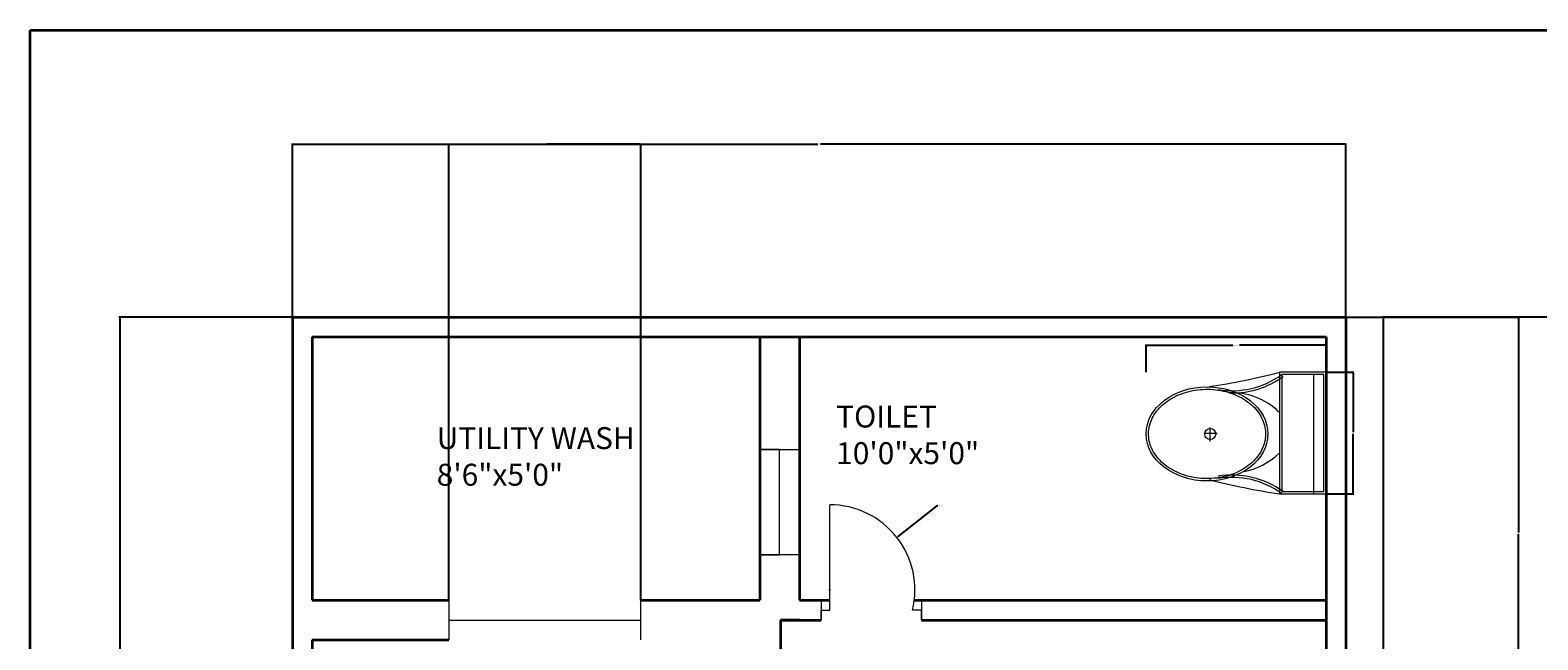
# Model space of a CAD drawing. Units: inches. Extents: x 1734 to 2405, y 1500 to 2491.
# Tile 13 of 14: x 1734 to 2078, y 2352 to 2491. Entities that reach past the tile are written whole.
import ezdxf

# ---------------------------------------------------------------- set-up
doc = ezdxf.new("R2010")
doc.units = ezdxf.units.IN
for name, color, linetype, lineweight in [('A-ANNO-DIMS', 2, 'Continuous', 18), ('A-ANNO-TTLB', 7, 'Continuous', 35), ('A-AREA-IDEN', 7, 'Continuous', 18), ('A-DOOR', 3, 'Continuous', 18), ('A-FLOR-FIXT', 9, 'Continuous', 18), ('A-GLAZ', 4, 'Continuous', 18), ('A-WALL', 7, 'Continuous', 35)]:
    doc.layers.add(name, color=color, linetype=linetype, lineweight=lineweight)
doc.styles.get("Standard").update_dxf_attribs({"font": 'arial.ttf'})
doc.dimstyles.get("Standard").update_dxf_attribs({"dimtxt": 0.18, "dimasz": 0.18, "dimexe": 0.18, "dimexo": 0.0625, "dimgap": 0.09, "dimtad": 0, "dimtih": 1, "dimtoh": 1, "dimdec": 4, "dimzin": 0, "dimdsep": 46, "dimtxsty": 'Standard', "dimcen": 0.09, "dimadec": 0, "dimazin": 0, "dimtfac": 1, "dimtdec": 4, "dimtofl": 0, "dimtmove": 0, "dimatfit": 3, "dimfxl": 1, "dimtolj": 1, "dimtzin": 0, "dimarcsym": 0})

# ---------------------------------------------------------------- blocks, each defined once
blk = doc.blocks.new('A$C31115884')
for p, q in [((257.5, 466.4), (257.5, 523.2)), ((283.1, 497.7), (223.4, 497.7)), ((0, 200), (0, 0)), ((520, 200), (0, 200)), ((520, 0), (520, 200)), ((10, 190), (10, 10)), ((510, 190), (10, 190)), ((510, 10), (510, 190)), ((510, 54.5), (0, 54.5)), ((10, 10), (510, 10)), ((0, 0), (520, 0))]:
    blk.add_line(p, q)
blk.add_circle((255.6, 496.4), 23.6)
for centre, radius, start, end in [((2777.7, -204.6), 2807, 165.4549, 171.71327), ((-294.5, 403.3), 364.7, 324.20913, 9.34987), ((-294.5, 403.3), 374.7, 324.20913, 9.34987), ((805.8, 403.3), 364.7, 170.65013, 215.79087), ((3237, 905), 2807, 188.28673, 194.5451), ((139.5, 406.2), 293.5, 315.84364, 2.65635), ((805.8, 403.3), 374.7, 179.20365, 215.79087), ((383.6, 406.2), 293.5, 190.27735, 224.15636)]:
    blk.add_arc(centre, radius, start, end)
blk.add_ellipse((256.2, 509.9), major_axis=(0, -260.7), ratio=0.772727)
blk.add_open_spline([(256.2, 259.2), (263.1, 259.2), (270, 259.7), (287.8, 262.3), (298.7, 265.1), (319.9, 273.1), (330.2, 278.4), (350.1, 291.1), (359.7, 298.7), (377.7, 315.9), (386.2, 325.5), (401.7, 346.6), (408.8, 358.1), (421.3, 382.5), (426.8, 395.5), (435.9, 422.4), (439.5, 436.4), (444.8, 465.1), (446.5, 479.7), (447.9, 509.2), (447.6, 524), (445, 553.3), (442.7, 567.8), (436.3, 596), (432.1, 609.7), (421.9, 636), (416, 648.6), (402.5, 672.1), (395, 683), (378.6, 703), (369.8, 712.1), (351.1, 728), (341.3, 734.8), (320.9, 746.2), (310.4, 750.7), (288.9, 757.3), (278, 759.4), (256, 761), (245, 760.6), (223.1, 757.2), (212.3, 754.3), (191.1, 746.1), (180.8, 740.7), (160.9, 727.8), (151.4, 720.1), (133.5, 702.7), (125.1, 693), (109.6, 671.7), (102.6, 660.2), (90.2, 635.7), (84.9, 622.7), (76, 595.6), (72.4, 581.6), (67.2, 552.9), (65.6, 538.2), (64.4, 508.8), (64.8, 494), (67.5, 464.7), (69.9, 450.2), (76.6, 422), (80.8, 408.3), (91.1, 382.2), (97.2, 369.7), (110.8, 346.3), (118.4, 335.4), (134.8, 315.6), (143.7, 306.7), (162.4, 290.9), (172.3, 284.2), (192.8, 273), (203.3, 268.6), (224.8, 262.2), (235.8, 260.2), (249.9, 259.3), (253, 259.2), (256.2, 259.2)], degree=3, knots=[0, 0, 0, 0, 0.110105, 0.110105, 0.285049, 0.285049, 0.459994, 0.459994, 0.634938, 0.634938, 0.809882, 0.809882, 0.984827, 0.984827, 1.159771, 1.159771, 1.334715, 1.334715, 1.50966, 1.50966, 1.684604, 1.684604, 1.859549, 1.859549, 2.034493, 2.034493, 2.209437, 2.209437, 2.384382, 2.384382, 2.559326, 2.559326, 2.73427, 2.73427, 2.909215, 2.909215, 3.084159, 3.084159, 3.259103, 3.259103, 3.434048, 3.434048, 3.608992, 3.608992, 3.783936, 3.783936, 3.958881, 3.958881, 4.133825, 4.133825, 4.30877, 4.30877, 4.483714, 4.483714, 4.658658, 4.658658, 4.833603, 4.833603, 5.008547, 5.008547, 5.183491, 5.183491, 5.358436, 5.358436, 5.53338, 5.53338, 5.708324, 5.708324, 5.883269, 5.883269, 6.058213, 6.058213, 6.233158, 6.233158, 6.283185, 6.283185, 6.283185, 6.283185])
blk = doc.blocks.new('*D8')
at = {"layer": 'A-ANNO-DIMS', "color": 0, "lineweight": -2, "transparency": 16777216}
for p, q in [((1988.42, 2413.29), (1988.42, 2419.56)), ((1988.6, 2419.38), (2008.13, 2419.38)), ((2029.21, 2419.38), (2009.68, 2419.38)), ((2029.39, 2413.29), (2029.39, 2419.56))]:
    blk.add_line(p, q, dxfattribs=at)
at = {"layer": 'A-ANNO-DIMS', "color": 0, "transparency": 16777216}
for points in [[(1988.6, 2419.41), (1988.6, 2419.35), (1988.42, 2419.38)], [(2029.21, 2419.41), (2029.21, 2419.35), (2029.39, 2419.38)]]:
    blk.add_solid(points, dxfattribs=at)
at = {"layer": 'Defpoints', "color": 0, "transparency": 16777216}
for p in [(1988.42, 2419.38), (1988.42, 2413.23), (2029.39, 2413.23)]:
    blk.add_point(p, dxfattribs=at)
at = {"layer": 'A-ANNO-DIMS', "color": 0, "transparency": 16777216, "insert": (2008.91, 2419.38), "char_height": 0.18, "attachment_point": 5}
blk.add_mtext('\\A1;WC 41 TYP.', dxfattribs=at)
blk = doc.blocks.new('*D9')
at = {"layer": 'A-ANNO-DIMS', "color": 0, "lineweight": -2, "transparency": 16777216}
for p, q in [((2029.46, 2413.23), (2035.72, 2413.23)), ((2035.54, 2413.05), (2035.54, 2399.59)), ((2035.54, 2385.76), (2035.54, 2399.22)), ((2029.46, 2385.58), (2035.72, 2385.58))]:
    blk.add_line(p, q, dxfattribs=at)
at = {"layer": 'A-ANNO-DIMS', "color": 0, "transparency": 16777216}
for points in [[(2035.51, 2413.05), (2035.57, 2413.05), (2035.54, 2413.23)], [(2035.51, 2385.76), (2035.57, 2385.76), (2035.54, 2385.58)]]:
    blk.add_solid(points, dxfattribs=at)
at = {"layer": 'Defpoints', "color": 0, "transparency": 16777216}
for p in [(2029.39, 2413.23), (2035.54, 2413.23), (2029.39, 2385.58)]:
    blk.add_point(p, dxfattribs=at)
at = {"layer": 'A-ANNO-DIMS', "color": 0, "transparency": 16777216, "insert": (2035.54, 2399.4), "char_height": 0.18, "attachment_point": 5}
blk.add_mtext('\\A1;28 TYP.', dxfattribs=at)
blk = doc.blocks.new('*D22')
at = {"layer": 'A-ANNO-DIMS', "color": 0, "lineweight": -2, "transparency": 16777216}
for p, q in [((1793.89, 2425.89), (1793.89, 2465.35)), ((1794.07, 2465.17), (1913.6, 2465.17)), ((2033.71, 2465.17), (1914.18, 2465.17)), ((2033.89, 2425.89), (2033.89, 2465.35))]:
    blk.add_line(p, q, dxfattribs=at)
at = {"layer": 'A-ANNO-DIMS', "color": 0, "transparency": 16777216}
for points in [[(1794.07, 2465.2), (1794.07, 2465.14), (1793.89, 2465.17)], [(2033.71, 2465.2), (2033.71, 2465.14), (2033.89, 2465.17)]]:
    blk.add_solid(points, dxfattribs=at)
at = {"layer": 'Defpoints', "color": 0, "transparency": 16777216}
for p in [(2033.89, 2465.17), (1793.89, 2425.82), (2033.89, 2425.82)]:
    blk.add_point(p, dxfattribs=at)
at = {"layer": 'A-ANNO-DIMS', "color": 0, "transparency": 16777216, "insert": (1913.89, 2465.17), "char_height": 0.18, "attachment_point": 5}
blk.add_mtext('\\A1;240', dxfattribs=at)
blk = doc.blocks.new('*D23')
at = {"layer": 'A-ANNO-DIMS', "color": 0, "lineweight": -2, "transparency": 16777216}
for p, q in [((1793.83, 2425.82), (1754.36, 2425.82)), ((1754.54, 2425.64), (1754.54, 2068.48)), ((1754.54, 1710.95), (1754.54, 2068.11)), ((1793.83, 1710.77), (1754.36, 1710.77))]:
    blk.add_line(p, q, dxfattribs=at)
at = {"layer": 'A-ANNO-DIMS', "color": 0, "transparency": 16777216}
for points in [[(1754.51, 2425.64), (1754.57, 2425.64), (1754.54, 2425.82)], [(1754.51, 1710.95), (1754.57, 1710.95), (1754.54, 1710.77)]]:
    blk.add_solid(points, dxfattribs=at)
at = {"layer": 'Defpoints', "color": 0, "transparency": 16777216}
for p in [(1754.54, 2425.82), (1793.89, 2425.82), (1793.89, 1710.77)]:
    blk.add_point(p, dxfattribs=at)
at = {"layer": 'A-ANNO-DIMS', "color": 0, "transparency": 16777216, "insert": (1754.54, 2068.3), "char_height": 0.18, "attachment_point": 5}
blk.add_mtext('\\A1;715', dxfattribs=at)
blk = doc.blocks.new('*D30')
at = {"layer": 'A-ANNO-DIMS', "color": 0, "lineweight": -2, "transparency": 16777216}
for p, q in [((2033.96, 2425.82), (2073.42, 2425.82)), ((2073.24, 2425.64), (2073.24, 2376.77)), ((2073.24, 2327.53), (2073.24, 2376.41)), ((2033.96, 2327.35), (2073.42, 2327.35))]:
    blk.add_line(p, q, dxfattribs=at)
at = {"layer": 'A-ANNO-DIMS', "color": 0, "transparency": 16777216}
for points in [[(2073.21, 2425.64), (2073.27, 2425.64), (2073.24, 2425.82)], [(2073.21, 2327.53), (2073.27, 2327.53), (2073.24, 2327.35)]]:
    blk.add_solid(points, dxfattribs=at)
at = {"layer": 'Defpoints', "color": 0, "transparency": 16777216}
for p in [(2033.89, 2425.82), (2073.24, 2425.82), (2033.89, 2327.35)]:
    blk.add_point(p, dxfattribs=at)
at = {"layer": 'A-ANNO-DIMS', "color": 0, "transparency": 16777216, "insert": (2073.24, 2376.59), "char_height": 0.18, "attachment_point": 5}
blk.add_mtext('\\A1;98.47', dxfattribs=at)
blk = doc.blocks.new('*D31')
at = {"layer": 'A-ANNO-DIMS', "color": 0, "lineweight": -2, "transparency": 16777216}
for p, q in [((1829.55, 2361.39), (1829.55, 2465.35)), ((1829.73, 2465.17), (1851.02, 2465.17)), ((1873.12, 2465.17), (1851.82, 2465.17)), ((1873.3, 2361.39), (1873.3, 2465.35))]:
    blk.add_line(p, q, dxfattribs=at)
at = {"layer": 'A-ANNO-DIMS', "color": 0, "transparency": 16777216}
for points in [[(1829.73, 2465.2), (1829.73, 2465.14), (1829.55, 2465.17)], [(1873.12, 2465.2), (1873.12, 2465.14), (1873.3, 2465.17)]]:
    blk.add_solid(points, dxfattribs=at)
at = {"layer": 'Defpoints', "color": 0, "transparency": 16777216}
for p in [(1873.3, 2465.17), (1829.55, 2361.32), (1873.3, 2361.32)]:
    blk.add_point(p, dxfattribs=at)
at = {"layer": 'A-ANNO-DIMS', "color": 0, "transparency": 16777216, "insert": (1851.42, 2465.17), "char_height": 0.18, "attachment_point": 5}
blk.add_mtext('\\A1;43.75', dxfattribs=at)
blk = doc.blocks.new('*D36')
at = {"layer": 'A-ANNO-DIMS', "color": 0, "lineweight": -2, "transparency": 16777216}
for p, q in [((2081.68, 2425.82), (2042.21, 2425.82)), ((2042.39, 2425.64), (2042.39, 2065.96)), ((2042.39, 1705.92), (2042.39, 2065.6)), ((2081.68, 1705.74), (2042.21, 1705.74))]:
    blk.add_line(p, q, dxfattribs=at)
at = {"layer": 'A-ANNO-DIMS', "color": 0, "transparency": 16777216}
for points in [[(2042.36, 2425.64), (2042.42, 2425.64), (2042.39, 2425.82)], [(2042.36, 1705.92), (2042.42, 1705.92), (2042.39, 1705.74)]]:
    blk.add_solid(points, dxfattribs=at)
at = {"layer": 'Defpoints', "color": 0, "transparency": 16777216}
for p in [(2042.39, 2425.82), (2081.74, 2425.82), (2081.74, 1705.74)]:
    blk.add_point(p, dxfattribs=at)
at = {"layer": 'A-ANNO-DIMS', "color": 0, "transparency": 16777216, "insert": (2042.39, 2065.78), "char_height": 0.18, "attachment_point": 5}
blk.add_mtext('\\A1;720.1', dxfattribs=at)
blk = doc.blocks.new('*D49')
at = {"layer": 'A-ANNO-DIMS', "color": 0, "lineweight": -2, "transparency": 16777216}
for p, q in [((1940.74, 2382.85), (1931.73, 2375.77)), ((1940.92, 2382.85), (1940.74, 2382.85)), ((1916.23, 2363.67), (1916.41, 2363.67)), ((1916.32, 2363.58), (1916.32, 2363.76))]:
    blk.add_line(p, q, dxfattribs=at)
at = {"layer": 'A-ANNO-DIMS', "color": 0, "transparency": 16777216}
blk.add_solid([(1931.71, 2375.79), (1931.74, 2375.74), (1931.58, 2375.66)], dxfattribs=at)
at = {"layer": 'Defpoints', "color": 0, "transparency": 16777216}
for p in [(1931.58, 2375.66), (1916.32, 2363.67)]:
    blk.add_point(p, dxfattribs=at)
at = {"layer": 'A-ANNO-DIMS', "color": 0, "transparency": 16777216, "insert": (1941.38, 2382.85), "char_height": 0.18, "attachment_point": 5}
blk.add_mtext('\\A1;R19.41', dxfattribs=at)

msp = doc.modelspace()

# ---------------------------------------------------------------- linework, layer by layer
at = {"layer": 'A-ANNO-TTLB'}
msp.add_lwpolyline([(1734.1307, 2491.1293), (2404.5589, 2491.1293), (2404.5589, 1500.293), (1734.1307, 1500.293)], close=True, dxfattribs=at)
at = {"layer": 'A-DOOR'}
for p, q in [((1916.3223, 2359.0746), (1916.3223, 2383.0746)), ((1914.3223, 2361.3246), (1914.3223, 2356.8246)), ((1937.1806, 2361.3246), (1937.1806, 2356.8246)), ((1914.3223, 2356.8246), (1914.3223, 2359.0746)), ((1914.3223, 2359.0746), (1916.3223, 2359.0746)), ((1937.1806, 2359.0746), (1935.1806, 2359.0746)), ((1937.1806, 2356.8246), (1937.1806, 2359.0746))]:
    msp.add_line(p, q, dxfattribs=at)
msp.add_arc((1916.3223, 2363.6655), 19.4091, 346.317899, 90, dxfattribs=at)
at = {"layer": 'A-GLAZ'}
for p, q in [((1904.8942, 2395.678), (1900.3942, 2395.678)), ((1900.3942, 2395.678), (1900.3942, 2395.678)), ((1900.3942, 2395.678), (1909.3942, 2395.678)), ((1904.8942, 2371.678), (1904.8942, 2395.678)), ((1909.3942, 2371.678), (1900.3942, 2371.678)), ((1900.3942, 2371.678), (1904.8942, 2371.678)), ((1829.5495, 2361.3246), (1829.5495, 2352.3246)), ((1873.2951, 2352.3246), (1873.2951, 2361.3246)), ((1829.5495, 2356.8246), (1873.2951, 2356.8246))]:
    msp.add_line(p, q, dxfattribs=at)
at = {"layer": 'A-WALL'}
for p, q in [((1793.8942, 2425.8246), (2033.8942, 2425.8246)), ((1793.8942, 2425.8246), (1793.8942, 1891.8246)), ((2033.8942, 2425.8246), (2033.8942, 1798.8246)), ((1798.3942, 2421.3246), (2029.3942, 2421.3246)), ((1798.3942, 2421.3246), (1798.3942, 2361.3246)), ((1900.3942, 2421.3246), (1900.3942, 2361.3246)), ((1909.3942, 2421.3246), (1909.3942, 2361.3246)), ((2029.3942, 2421.3246), (2029.3942, 2206.8246)), ((1798.3942, 2361.3246), (1829.5495, 2361.3246)), ((1873.2951, 2361.3246), (1900.3942, 2361.3246)), ((1909.3942, 2361.3246), (1916.3223, 2361.3246)), ((1935.5897, 2361.3246), (2029.3942, 2361.3246)), ((1909.3942, 2356.8246), (1905.0875, 2356.8246)), ((1905.0875, 2356.8246), (1905.0875, 2206.8246)), ((1905.0875, 2356.8246), (1914.3223, 2356.8246)), ((1937.1806, 2356.8246), (2029.3942, 2356.8246)), ((1798.3942, 2352.3246), (1829.5495, 2352.3246)), ((1798.3942, 2352.3246), (1798.3942, 2206.8246))]:
    msp.add_line(p, q, dxfattribs=at)

# ---------------------------------------------------------------- block references
at = {"layer": 'A-FLOR-FIXT', "xscale": 0.0531771398825126, "yscale": 0.0531771398825126, "zscale": 0.0531771398825126, "rotation": 89.99999999999999}
msp.add_blockref('A$C31115884', (2029.3942, 2385.5788), dxfattribs=at)

# ---------------------------------------------------------------- texts
at = {"layer": 'A-AREA-IDEN', "char_height": 5, "attachment_point": 1}
for s, width, insert in [('TOILET\\P10\'0"x5\'0"', 172.59145, (1917.7724, 2405.66)), ('UTILITY WASH\\P8\'6"x5\'0"', 145.633739, (1826.7657, 2400.7415))]:
    msp.add_mtext_dynamic_manual_height_columns(s, width=width, gutter_width=12.5, heights=[0], dxfattribs=dict(at, insert=insert))

# ---------------------------------------------------------------- dimensions: what is measured, and where the dimension line sits
at = {"layer": 'A-ANNO-DIMS'}
for base, p1, p2, override, picture, middle in [((2033.8942, 2465.1746), (1793.8942, 2425.8246), (2033.8942, 2425.8246), {"dimdec": 0, "dimlfac": 1, "dimrnd": 0, "dimzin": 0, "dimdsep": 46, "dimlunit": 2}, '*D22', (1913.8942, 2465.1746)), ((1873.2951, 2465.1746), (1829.5495, 2361.3246), (1873.2951, 2361.3246), {"dimdec": 2, "dimlfac": 1, "dimrnd": 0, "dimzin": 0, "dimdsep": 46, "dimlunit": 2}, '*D31', (1851.4223, 2465.1746))]:
    dim = msp.add_linear_dim(base=base, p1=p1, p2=p2, dimstyle='Standard', override=override, dxfattribs=at)
    dim.commit()
    dim.dimension.update_dxf_attribs({"geometry": picture, "text_midpoint": middle})
for base, p1, p2, override, picture, middle in [((1754.5442, 2425.8246), (1793.8942, 1710.7667), (1793.8942, 2425.8246), {"dimdec": 0, "dimlfac": 1, "dimrnd": 0, "dimzin": 0, "dimdsep": 46, "dimlunit": 2}, '*D23', (1754.5442, 2068.2956)), ((2073.2442, 2425.8246), (2033.8942, 2327.351), (2033.8942, 2425.8246), {"dimdec": 2, "dimlfac": 1, "dimrnd": 0, "dimzin": 0, "dimdsep": 46, "dimlunit": 2}, '*D30', (2073.2442, 2376.5878)), ((2042.3945, 2425.8246), (2081.7445, 1705.7415), (2081.7445, 2425.8246), {"dimdec": 1, "dimlfac": 1, "dimrnd": 0, "dimzin": 0, "dimdsep": 46, "dimlunit": 2}, '*D36', (2042.3945, 2065.783))]:
    dim = msp.add_linear_dim(base=base, p1=p1, p2=p2, angle=90, dimstyle='Standard', override=override, dxfattribs=at)
    dim.commit()
    dim.dimension.update_dxf_attribs({"geometry": picture, "text_midpoint": middle})
for base, p1, p2, angle, text, picture, middle in [((1988.4175, 2419.3774), (2029.3942, 2413.2309), (1988.4175, 2413.2309), 180, 'WC <> TYP.', '*D8', (2008.9058, 2419.3774)), ((2035.5407, 2413.2309), (2029.3942, 2385.5788), (2029.3942, 2413.2309), 90, '<> TYP.', '*D9', (2035.5407, 2399.4048))]:
    dim = msp.add_linear_dim(base=base, p1=p1, p2=p2, angle=angle, text=text, dimstyle='Standard', override={"dimdec": 0, "dimlfac": 1, "dimrnd": 0, "dimzin": 0, "dimdsep": 46, "dimlunit": 2}, dxfattribs=at)
    dim.commit()
    dim.dimension.update_dxf_attribs({"geometry": picture, "text_midpoint": middle})
dim = msp.add_radius_dim(center=(1916.3223, 2363.6655), mpoint=(1931.5839, 2375.657), dimstyle='Standard', override={"dimdec": 2, "dimlfac": 1, "dimrnd": 0, "dimzin": 0, "dimdsep": 46, "dimlunit": 2}, dxfattribs=at)
dim.commit()
dim.dimension.update_dxf_attribs({"geometry": '*D49', "text_midpoint": (1941.3834, 2382.8518), "dimtype": 164})

doc.saveas('drawing.dxf')
